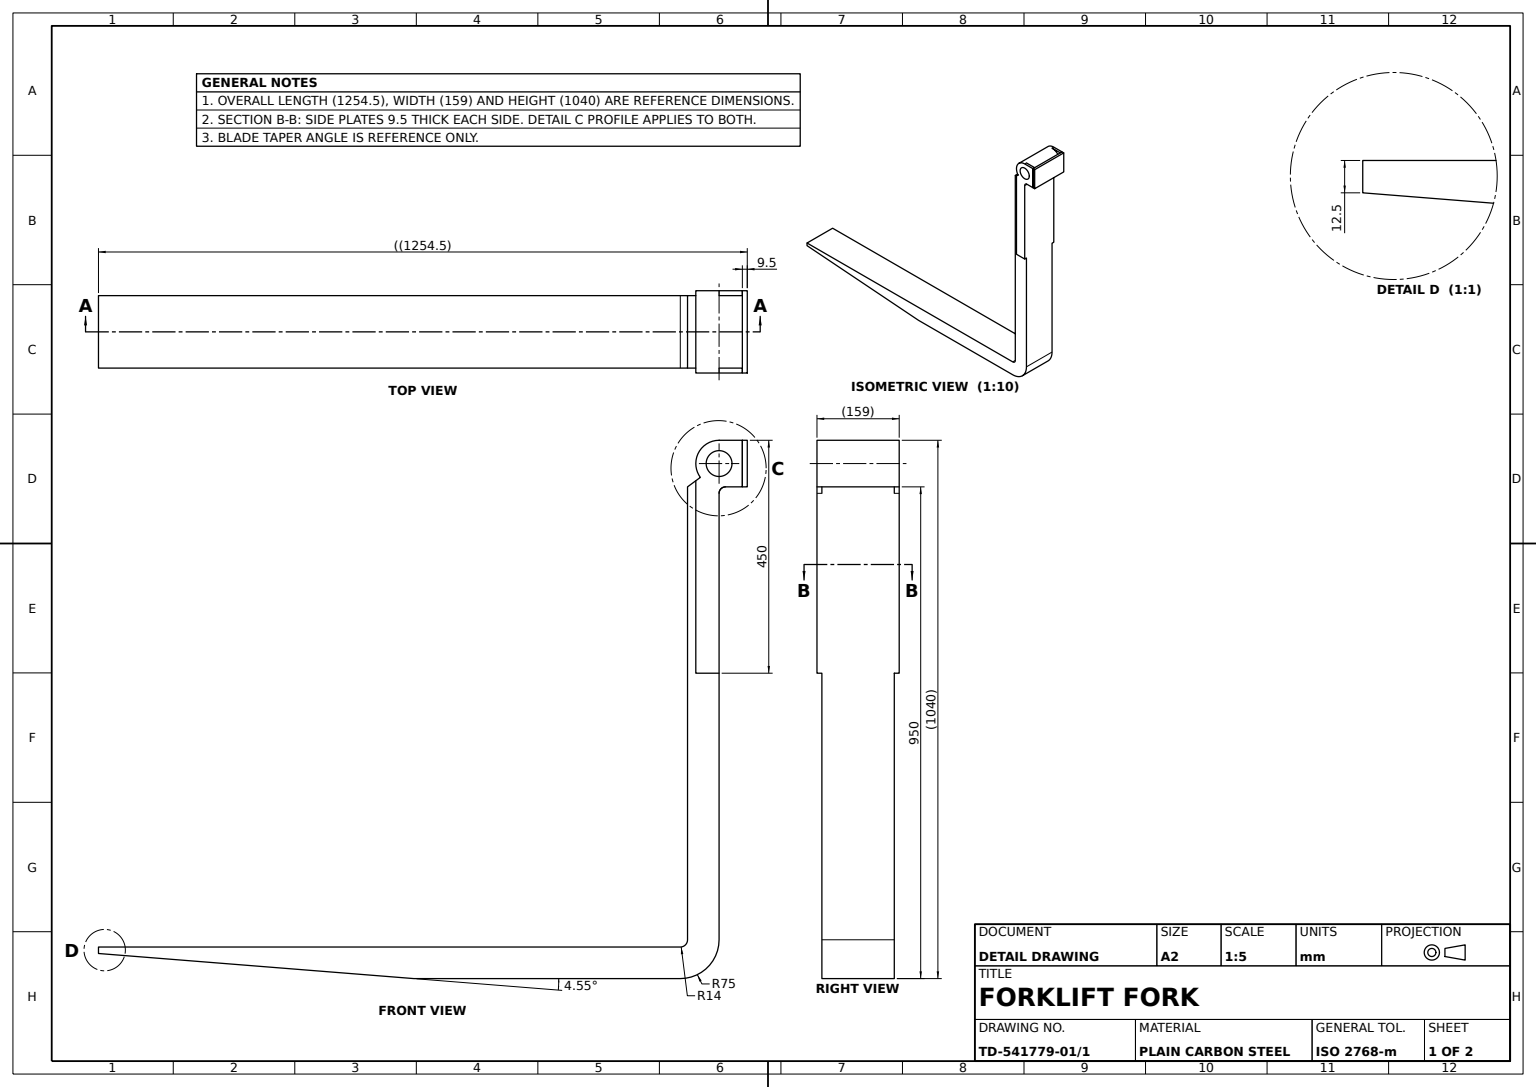
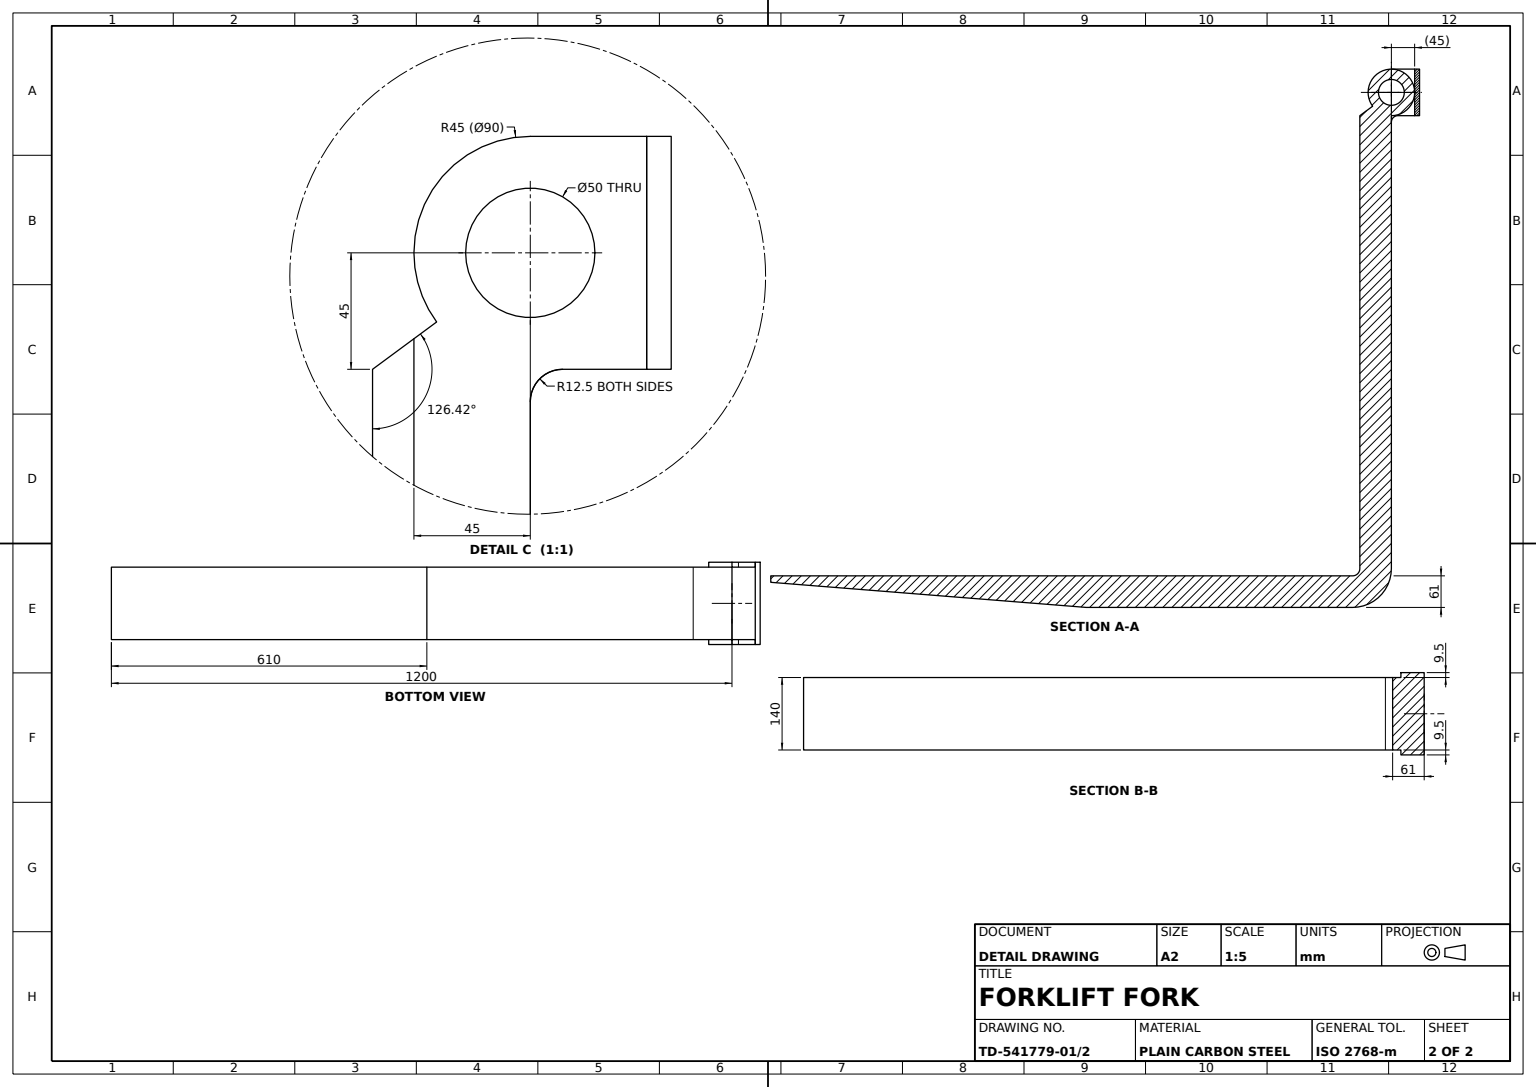
from build123d import *
from build123d.topology import SkipClean

# Parameters (mm, degrees)
FORK_BLADE_AND_SHANK_DEPTH     = 70
BLADE_TIP_TAPER_CUT_DEPTH      = 1537.912489376
BLADE_TIP_TAPER_CUT_DEPTH_BACK = 1537.912489376
SHANK_BOSS_SKETCH_R            = 45
SHANK_BOSS_SKETCH_R_2          = 25
SHANK_LOWER_BOSS_DEPTH         = 70
SHANK_UPPER_BOSS_DEPTH         = 70
SIDE_START                     = 9.5
SIDE_PLATE_SKETCH_R            = 25
SIDE_PLATE_DEPTH               = 9.5
TOP_HOOK_BLOCK_SKETCH_W        = 159
TOP_HOOK_BLOCK_SKETCH_H        = 90
TOP_HOOK_BLOCK_DEPTH           = 9.5


with BuildPart() as part:
    # Fork L-Profile Sketch → Fork Blade and Shank (new, symmetric)
    with BuildSketch(Plane.XY):
        with BuildLine():
            Line((0, 950), (0, 75))
            ThreePointArc((0, 75), (-21.966991411, 21.966991411), (-75, 0))
            Line((-75, 0), (-1200, 0))
            Line((-1200, 0), (-1200, 61))
            Line((-1200, 61), (-75, 61))
            ThreePointArc((-75, 61), (-65.100505063, 65.100505063), (-61, 75))
            Line((-61, 75), (-61, 950))
            Line((-61, 950), (0, 950))
        make_face()
    extrude(amount=FORK_BLADE_AND_SHANK_DEPTH, both=True)

    # Blade Taper Sketch → Blade Tip Taper Cut (cut, two sides: drawn at the far end of the back side and taken through both)
    with BuildSketch(Plane.XY.offset(70).offset(-BLADE_TIP_TAPER_CUT_DEPTH_BACK)):
        Polygon((-4202.326226889, 287.209544269), (-1200, 48.5), (-590, 0), (2412.326226889, -238.709544269), (1934.907138351, -6243.361998046), (-4679.745315427, -5717.442909508), align=None)
    extrude(amount=BLADE_TIP_TAPER_CUT_DEPTH + BLADE_TIP_TAPER_CUT_DEPTH_BACK, mode=Mode.SUBTRACT)



with BuildPart() as body_2:
    # Shank Boss Sketch → Shank Lower Boss (new, symmetric)
    with BuildSketch(Plane.XY):
        with Locations((0, 995)):
            Circle(SHANK_BOSS_SKETCH_R)
        with Locations((0, 995)):
            Circle(SHANK_BOSS_SKETCH_R_2, mode=Mode.SUBTRACT)
    extrude(amount=SHANK_LOWER_BOSS_DEPTH, both=True)


with BuildPart() as part_1:
    add(part.part)

    add(body_2.part)  # Shank Upper Boss merges body 2
    # Shank Upper Boss Sketch → Shank Upper Boss (add, symmetric)
    with BuildSketch(Plane.XY):
        with BuildLine():
            Line((-36.212585863, 968.285797314), (-61, 950))
            Line((-61, 950), (0, 950))
            ThreePointArc((0, 950), (-20.283748164, 954.830738612), (-36.212585863, 968.285797314))
        make_face()
    extrude(amount=SHANK_UPPER_BOSS_DEPTH, both=True)

    # Side Plate Sketch → Side Plate (add)
    # profile 1 of 4: a face of its own
    with BuildSketch(Plane.XY.offset(70).offset(SIDE_START)):
        with BuildLine():
            Line((45, 1040), (0, 1040))
            ThreePointArc((0, 1040), (31.819805153, 1026.819805153), (45, 995))
            Line((45, 995), (45, 1040))
        make_face()
    # profile 2 of 4: a face of its own
    with BuildSketch(Plane.XY.offset(70).offset(SIDE_START)):
        with BuildLine():
            Line((45, 950), (45, 995))
            ThreePointArc((45, 995), (31.819805153, 963.180194847), (0, 950))
            Line((0, 950), (0, 937.5))
            ThreePointArc((0, 937.5), (3.661165235, 946.338834765), (12.5, 950))
            Line((12.5, 950), (45, 950))
        make_face()
    # profile 3 of 4: a face of its own
    with BuildSketch(Plane.XY.offset(70).offset(SIDE_START)):
        with BuildLine():
            ThreePointArc((0, 1040), (-31.819805153, 1026.819805153), (-45, 995))
            ThreePointArc((-45, 995), (-42.746732997, 980.938818752), (-36.212585863, 968.285797314))
            Line((-36.212585863, 968.285797314), (-45, 961.803278689))
            Line((-45, 961.803278689), (-45, 950))
            Line((-45, 950), (0, 950))
            ThreePointArc((0, 950), (31.819805153, 963.180194847), (45, 995))
            ThreePointArc((45, 995), (31.819805153, 1026.819805153), (0, 1040))
        make_face()
        with Locations((0, 995)):
            Circle(SIDE_PLATE_SKETCH_R, mode=Mode.SUBTRACT)
    # profile 4 of 4: a face of its own
    with BuildSketch(Plane.XY.offset(70).offset(SIDE_START)):
        Polygon((0, 950), (-45, 950), (-45, 590), (0, 590), (0, 937.5), align=None)
    side_plate = extrude(amount=-SIDE_PLATE_DEPTH)

    # Side Plate Mirror: Side Plate across plane
    with SkipClean():  # the faces are left unmerged after this step: merging them gives an invalid solid
        add(side_plate.mirror(Plane.XY))


with BuildPart() as body_2_2:
    # Top Hook Block Sketch → Top Hook Block (new body)
    with BuildSketch(Plane(origin=(45, 0, 0), x_dir=(0, 0, -1), z_dir=(1, 0, 0))):
        with Locations((0, 995)):
            Rectangle(TOP_HOOK_BLOCK_SKETCH_W, TOP_HOOK_BLOCK_SKETCH_H)
    extrude(amount=TOP_HOOK_BLOCK_DEPTH)


solid = Compound([part_1.part, body_2_2.part])
